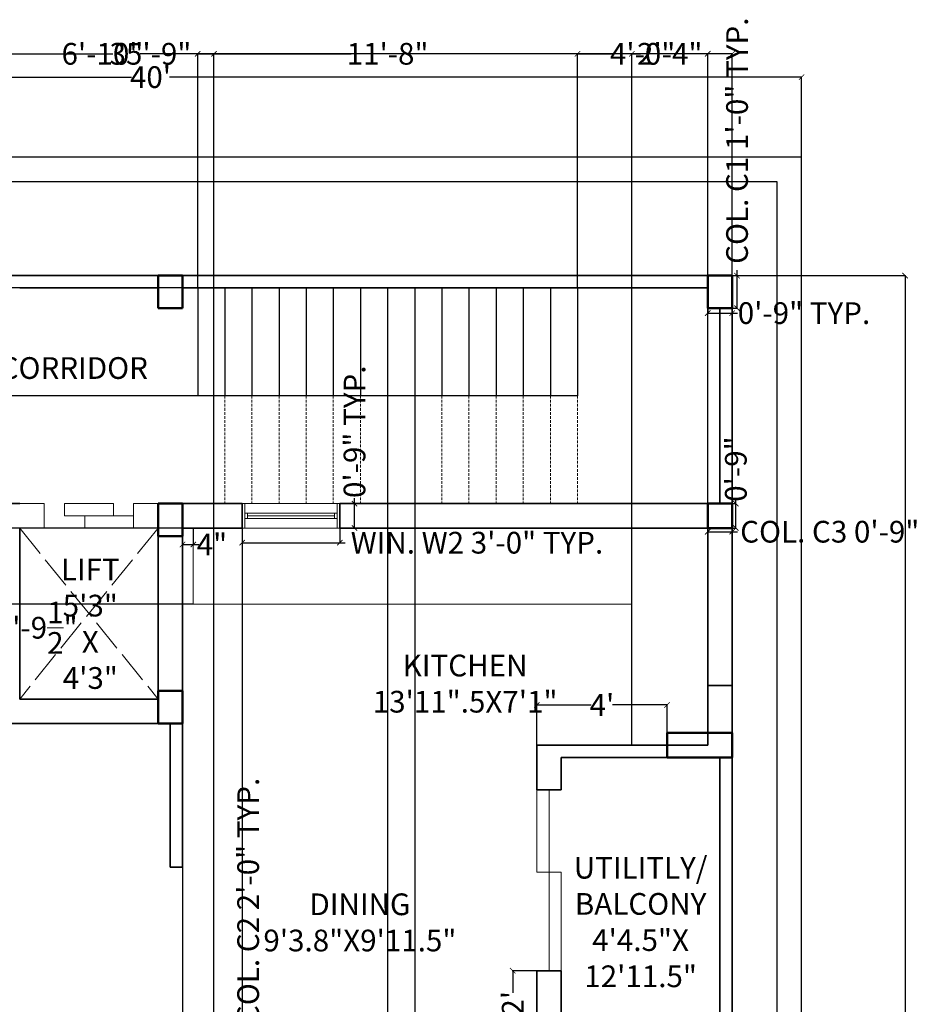
# Model space of a CAD drawing. Units: inches. Extents: x 490 to 1091, y 501 to 1322.
# Tile 5 of 5: x 759 to 1091, y 959 to 1322. Entities that reach past the tile are written whole.
import ezdxf

# ---------------------------------------------------------------- set-up
doc = ezdxf.new("R2010")
doc.units = ezdxf.units.IN
doc.header["$MEASUREMENT"] = 0
doc.linetypes.add('ACAD_ISO02W100', pattern=[15, 12, -3])
doc.linetypes.add('DASHEDX2', pattern=[1.5, 1, -0.5])
for name, color, linetype, lineweight in [('A-ANNO-DIMS', 2, 'Continuous', 18), ('A-AREA-IDEN', 7, 'Continuous', 25), ('A-COLS', 12, 'Continuous', 50), ('A-DOOR', 3, 'Continuous', 20), ('A-EQPM-EVTR', 152, 'Continuous', 20), ('A-EQPM-EVTR-HIDN', 152, 'ACAD_ISO02W100', 13), ('A-FLOR-FIXT', 8, 'Continuous', 20), ('A-FLOR-STRS', 12, 'Continuous', 25), ('A-FLOR-STRS-OVHD', 12, 'DASHEDX2', 18), ('A-GLAZ', 4, 'Continuous', 18), ('A-WALL', 7, 'Continuous', 35), ('C-PROP', 8, 'Continuous', 25)]:
    doc.layers.add(name, color=color, linetype=linetype, lineweight=lineweight)
doc.styles.get("Standard").update_dxf_attribs({"font": 'arial.ttf'})
doc.dimstyles.get("Standard").update_dxf_attribs({"dimtxt": 8, "dimasz": 2, "dimexe": 0.18, "dimexo": 0.0625, "dimgap": 0.09, "dimtad": 0, "dimdec": 1, "dimzin": 0, "dimdsep": 46, "dimlunit": 4, "dimtxsty": 'Standard', "dimblk": 'ARCHTICK', "dimcen": 0.09, "dimadec": 0, "dimazin": 0, "dimtfac": 1, "dimtdec": 1, "dimtofl": 0, "dimtmove": 0, "dimatfit": 3, "dimldrblk": 'ARCHTICK', "dimfxl": 1, "dimtolj": 1, "dimtzin": 0, "dimarcsym": 0})

# ---------------------------------------------------------------- blocks, each defined once
blk = doc.blocks.new('_ArchTick')
at = {"color": 0, "linetype": 'ByBlock', "const_width": 0.15}
blk.add_lwpolyline([(-0.5, -0.5), (0.5, 0.5)], dxfattribs=at)
blk = doc.blocks.new('*D3')
at = {"layer": 'A-ANNO-DIMS', "color": 0, "lineweight": -2, "transparency": 16777216}
for p, q in [((567.27, 1270.95), (567.27, 1300.61)), ((567.27, 1300.43), (800.23, 1300.43)), ((1047.27, 1300.43), (814.31, 1300.43)), ((1047.27, 1270.95), (1047.27, 1300.61))]:
    blk.add_line(p, q, dxfattribs=at)
at = {"layer": 'Defpoints', "color": 0, "transparency": 16777216}
for p in [(567.27, 1300.43), (567.27, 1270.88), (1047.27, 1270.88)]:
    blk.add_point(p, dxfattribs=at)
at = {"layer": 'A-ANNO-DIMS', "color": 0, "lineweight": -2, "transparency": 16777216, "xscale": 2, "yscale": 2, "zscale": 2, "rotation": 180}
blk.add_blockref('_ArchTick', (567.27, 1300.43), dxfattribs=at)
at = {"layer": 'A-ANNO-DIMS', "color": 0, "lineweight": -2, "transparency": 16777216, "xscale": 2, "yscale": 2, "zscale": 2}
blk.add_blockref('_ArchTick', (1047.27, 1300.43), dxfattribs=at)
at = {"layer": 'A-ANNO-DIMS', "color": 0, "transparency": 16777216, "insert": (807.27, 1300.43), "char_height": 8, "attachment_point": 5}
blk.add_mtext("\\A1;40'", dxfattribs=at)
blk = doc.blocks.new('jcjg  bmvh')
for p, q in [((1232.66, 1066.6), (1223.66, 1066.6)), ((1223.66, 1066.6), (1223.66, 1042.6)), ((1232.66, 1042.6), (1232.66, 1066.6)), ((1223.66, 1042.6), (1232.66, 1042.6))]:
    blk.add_line(p, q)
blk = doc.blocks.new('hcjfukik')
for p, q in [((1274.78, 1182.51), (1265.78, 1182.51)), ((1265.78, 1182.51), (1265.78, 1173.51)), ((1274.78, 1173.51), (1274.78, 1182.51)), ((1265.78, 1173.51), (1274.78, 1173.51))]:
    blk.add_line(p, q)
blk = doc.blocks.new('*D7')
at = {"layer": 'A-ANNO-DIMS', "color": 0, "lineweight": -2, "transparency": 16777216}
for p, q in [((949.67, 1054.35), (949.67, 1069.27)), ((949.67, 1069.09), (969.74, 1069.09)), ((997.67, 1069.09), (977.6, 1069.09)), ((997.67, 1054.35), (997.67, 1069.27))]:
    blk.add_line(p, q, dxfattribs=at)
at = {"layer": 'Defpoints', "color": 0, "transparency": 16777216}
for p in [(997.67, 1069.09), (949.67, 1054.28), (997.67, 1054.28)]:
    blk.add_point(p, dxfattribs=at)
at = {"layer": 'A-ANNO-DIMS', "color": 0, "lineweight": -2, "transparency": 16777216, "xscale": 2, "yscale": 2, "zscale": 2, "rotation": 180}
blk.add_blockref('_ArchTick', (949.67, 1069.09), dxfattribs=at)
at = {"layer": 'A-ANNO-DIMS', "color": 0, "lineweight": -2, "transparency": 16777216, "xscale": 2, "yscale": 2, "zscale": 2}
blk.add_blockref('_ArchTick', (997.67, 1069.09), dxfattribs=at)
at = {"layer": 'A-ANNO-DIMS', "color": 0, "transparency": 16777216, "insert": (973.67, 1069.09), "char_height": 8, "attachment_point": 5}
blk.add_mtext("\\A1;4'", dxfattribs=at)
blk = doc.blocks.new('*D13')
at = {"layer": 'A-ANNO-DIMS', "color": 0, "lineweight": -2, "transparency": 16777216}
for p, q in [((819.07, 1134.22), (819.07, 1128.05)), ((823.07, 1134.22), (823.07, 1128.05)), ((819.07, 1128.23), (823.07, 1128.23)), ((823.07, 1128.23), (825.07, 1128.23))]:
    blk.add_line(p, q, dxfattribs=at)
at = {"layer": 'Defpoints', "color": 0, "transparency": 16777216}
for p in [(819.07, 1134.28), (823.07, 1134.28), (823.07, 1128.23)]:
    blk.add_point(p, dxfattribs=at)
at = {"layer": 'A-ANNO-DIMS', "color": 0, "lineweight": -2, "transparency": 16777216, "xscale": 2, "yscale": 2, "zscale": 2, "rotation": 180}
blk.add_blockref('_ArchTick', (819.07, 1128.23), dxfattribs=at)
at = {"layer": 'A-ANNO-DIMS', "color": 0, "lineweight": -2, "transparency": 16777216, "xscale": 2, "yscale": 2, "zscale": 2}
blk.add_blockref('_ArchTick', (823.07, 1128.23), dxfattribs=at)
at = {"layer": 'A-ANNO-DIMS', "color": 0, "transparency": 16777216, "insert": (829.92, 1128.23), "char_height": 8, "attachment_point": 5}
blk.add_mtext('\\A1;4"', dxfattribs=at)
blk = doc.blocks.new('bnfgfhvhm')
for p, q in [((1106.43, 1203.63), (1115.43, 1203.63)), ((1106.43, 1191.63), (1106.43, 1203.63)), ((1115.43, 1203.63), (1115.43, 1191.63)), ((1115.43, 1191.63), (1106.43, 1191.63))]:
    blk.add_line(p, q)
blk = doc.blocks.new('fvbfbvc hbmh')
for p, q in [((1342.5, 1176.65), (1378.5, 1176.65)), ((1342.5, 1167.65), (1342.5, 1176.65)), ((1343.5, 1167.65), (1343.5, 1176.65)), ((1377.5, 1176.65), (1377.5, 1167.65)), ((1378.5, 1176.65), (1378.5, 1167.65)), ((1343.5, 1173.15), (1377.5, 1173.15)), ((1344.5, 1171.15), (1344.5, 1173.15)), ((1344.5, 1172.15), (1376.5, 1172.15)), ((1376.5, 1173.15), (1376.5, 1171.15)), ((1343.5, 1171.15), (1377.5, 1171.15)), ((1378.5, 1167.65), (1342.5, 1167.65))]:
    blk.add_line(p, q)
blk = doc.blocks.new('*D26')
at = {"layer": 'A-ANNO-DIMS', "color": 0, "lineweight": -2, "transparency": 16777216}
for p, q in [((728.47, 1134.22), (728.47, 1097.37)), ((750.07, 1134.22), (750.07, 1097.37)), ((728.47, 1097.55), (750.07, 1097.55)), ((750.07, 1097.55), (752.07, 1097.55))]:
    blk.add_line(p, q, dxfattribs=at)
at = {"layer": 'Defpoints', "color": 0, "transparency": 16777216}
for p in [(728.47, 1134.28), (750.07, 1134.28), (750.07, 1097.55)]:
    blk.add_point(p, dxfattribs=at)
at = {"layer": 'A-ANNO-DIMS', "color": 0, "lineweight": -2, "transparency": 16777216, "xscale": 2, "yscale": 2, "zscale": 2, "rotation": 180}
blk.add_blockref('_ArchTick', (728.47, 1097.55), dxfattribs=at)
at = {"layer": 'A-ANNO-DIMS', "color": 0, "lineweight": -2, "transparency": 16777216, "xscale": 2, "yscale": 2, "zscale": 2}
blk.add_blockref('_ArchTick', (750.07, 1097.55), dxfattribs=at)
at = {"layer": 'A-ANNO-DIMS', "color": 0, "transparency": 16777216, "insert": (765.33, 1097.55), "char_height": 8, "attachment_point": 5}
blk.add_mtext('\\A1;1\'-9{\\H1x;\\S1/2;}"', dxfattribs=at)
blk = doc.blocks.new('*D31')
at = {"layer": 'A-ANNO-DIMS', "color": 0, "lineweight": -2, "transparency": 16777216}
for p, q in [((949.61, 971.18), (940.6, 971.18)), ((940.78, 971.18), (940.78, 963.02)), ((940.78, 947.18), (940.78, 955.35)), ((949.61, 947.18), (940.6, 947.18))]:
    blk.add_line(p, q, dxfattribs=at)
at = {"layer": 'Defpoints', "color": 0, "transparency": 16777216}
for p in [(940.78, 971.18), (949.67, 971.18), (949.67, 947.18)]:
    blk.add_point(p, dxfattribs=at)
at = {"layer": 'A-ANNO-DIMS', "color": 0, "lineweight": -2, "transparency": 16777216, "xscale": 2, "yscale": 2, "zscale": 2}
for p, rotation in [((940.78, 971.18), 90), ((940.78, 947.18), 270)]:
    blk.add_blockref('_ArchTick', p, dxfattribs=dict(at, rotation=rotation))
at = {"layer": 'A-ANNO-DIMS', "color": 0, "transparency": 16777216, "insert": (940.78, 959.18), "char_height": 8, "attachment_point": 5, "rotation": 90}
blk.add_mtext("\\A1;2'", dxfattribs=at)
blk = doc.blocks.new('*D48')
at = {"layer": 'A-ANNO-DIMS', "color": 0, "lineweight": -2, "transparency": 16777216}
for p, q in [((1021.73, 1227.28), (1023.65, 1227.28)), ((1023.47, 1227.28), (1023.47, 1229.28)), ((1023.47, 1215.28), (1023.47, 1227.28)), ((1021.73, 1215.28), (1023.65, 1215.28))]:
    blk.add_line(p, q, dxfattribs=at)
at = {"layer": 'Defpoints', "color": 0, "transparency": 16777216}
for p in [(1021.67, 1227.28), (1023.47, 1227.28), (1021.67, 1215.28)]:
    blk.add_point(p, dxfattribs=at)
at = {"layer": 'A-ANNO-DIMS', "color": 0, "lineweight": -2, "transparency": 16777216, "xscale": 2, "yscale": 2, "zscale": 2}
for p, rotation in [((1023.47, 1227.28), 90), ((1023.47, 1215.28), 270)]:
    blk.add_blockref('_ArchTick', p, dxfattribs=dict(at, rotation=rotation))
at = {"layer": 'A-ANNO-DIMS', "color": 0, "transparency": 16777216, "insert": (1023.47, 1277), "char_height": 8, "attachment_point": 5, "rotation": 90}
blk.add_mtext('\\A1;COL. C1 1\'-0" TYP.', dxfattribs=at)
blk = doc.blocks.new('*D49')
at = {"layer": 'A-ANNO-DIMS', "color": 0, "lineweight": -2, "transparency": 16777216}
for p, q in [((1012.67, 1215.22), (1012.67, 1213.3)), ((1012.67, 1213.48), (1021.67, 1213.48)), ((1021.67, 1215.22), (1021.67, 1213.3)), ((1021.67, 1213.48), (1023.67, 1213.48))]:
    blk.add_line(p, q, dxfattribs=at)
at = {"layer": 'Defpoints', "color": 0, "transparency": 16777216}
for p in [(1012.67, 1215.28), (1021.67, 1215.28), (1021.67, 1213.48)]:
    blk.add_point(p, dxfattribs=at)
at = {"layer": 'A-ANNO-DIMS', "color": 0, "lineweight": -2, "transparency": 16777216, "xscale": 2, "yscale": 2, "zscale": 2, "rotation": 180}
blk.add_blockref('_ArchTick', (1012.67, 1213.48), dxfattribs=at)
at = {"layer": 'A-ANNO-DIMS', "color": 0, "lineweight": -2, "transparency": 16777216, "xscale": 2, "yscale": 2, "zscale": 2}
blk.add_blockref('_ArchTick', (1021.67, 1213.48), dxfattribs=at)
at = {"layer": 'A-ANNO-DIMS', "color": 0, "transparency": 16777216, "insert": (1048.14, 1213.48), "char_height": 8, "attachment_point": 5}
blk.add_mtext('\\A1;0\'-9" TYP.', dxfattribs=at)
blk = doc.blocks.new('*D50')
at = {"layer": 'A-ANNO-DIMS', "color": 0, "lineweight": -2, "transparency": 16777216}
for p, q in [((839.73, 947.18), (843.45, 947.18)), ((843.27, 947.18), (843.27, 949.18)), ((843.27, 923.18), (843.27, 947.18)), ((839.73, 923.18), (843.45, 923.18))]:
    blk.add_line(p, q, dxfattribs=at)
at = {"layer": 'Defpoints', "color": 0, "transparency": 16777216}
for p in [(839.67, 947.18), (843.27, 947.18), (839.67, 923.18)]:
    blk.add_point(p, dxfattribs=at)
at = {"layer": 'A-ANNO-DIMS', "color": 0, "lineweight": -2, "transparency": 16777216, "xscale": 2, "yscale": 2, "zscale": 2}
for p, rotation in [((843.27, 947.18), 90), ((843.27, 923.18), 270)]:
    blk.add_blockref('_ArchTick', p, dxfattribs=dict(at, rotation=rotation))
at = {"layer": 'A-ANNO-DIMS', "color": 0, "transparency": 16777216, "insert": (843.27, 996.9), "char_height": 8, "attachment_point": 5, "rotation": 90}
blk.add_mtext('\\A1;COL. C2 2\'-0" TYP.', dxfattribs=at)
blk = doc.blocks.new('*D52')
at = {"layer": 'A-ANNO-DIMS', "color": 0, "lineweight": -2, "transparency": 16777216}
for p, q in [((1012.67, 1134.22), (1012.67, 1132.75)), ((1012.67, 1132.93), (1021.67, 1132.93)), ((1021.67, 1134.22), (1021.67, 1132.75)), ((1021.67, 1132.93), (1023.67, 1132.93))]:
    blk.add_line(p, q, dxfattribs=at)
at = {"layer": 'Defpoints', "color": 0, "transparency": 16777216}
for p in [(1012.67, 1134.28), (1021.67, 1134.28), (1021.67, 1132.93)]:
    blk.add_point(p, dxfattribs=at)
at = {"layer": 'A-ANNO-DIMS', "color": 0, "lineweight": -2, "transparency": 16777216, "xscale": 2, "yscale": 2, "zscale": 2, "rotation": 180}
blk.add_blockref('_ArchTick', (1012.67, 1132.93), dxfattribs=at)
at = {"layer": 'A-ANNO-DIMS', "color": 0, "lineweight": -2, "transparency": 16777216, "xscale": 2, "yscale": 2, "zscale": 2}
blk.add_blockref('_ArchTick', (1021.67, 1132.93), dxfattribs=at)
at = {"layer": 'A-ANNO-DIMS', "color": 0, "transparency": 16777216, "insert": (1057.64, 1132.93), "char_height": 8, "attachment_point": 5}
blk.add_mtext('\\A1;COL. C3 0\'-9"', dxfattribs=at)
blk = doc.blocks.new('*D53')
at = {"layer": 'A-ANNO-DIMS', "color": 0, "lineweight": -2, "transparency": 16777216}
for p, q in [((1021.73, 1143.28), (1023.2, 1143.28)), ((1023.02, 1143.28), (1023.02, 1145.28)), ((1023.02, 1134.28), (1023.02, 1143.28)), ((1021.73, 1134.28), (1023.2, 1134.28))]:
    blk.add_line(p, q, dxfattribs=at)
at = {"layer": 'Defpoints', "color": 0, "transparency": 16777216}
for p in [(1021.67, 1143.28), (1023.02, 1143.28), (1021.67, 1134.28)]:
    blk.add_point(p, dxfattribs=at)
at = {"layer": 'A-ANNO-DIMS', "color": 0, "lineweight": -2, "transparency": 16777216, "xscale": 2, "yscale": 2, "zscale": 2}
for p, rotation in [((1023.02, 1143.28), 90), ((1023.02, 1134.28), 270)]:
    blk.add_blockref('_ArchTick', p, dxfattribs=dict(at, rotation=rotation))
at = {"layer": 'A-ANNO-DIMS', "color": 0, "transparency": 16777216, "insert": (1023.02, 1156.01), "char_height": 8, "attachment_point": 5, "rotation": 90}
blk.add_mtext('\\A1;0\'-9"', dxfattribs=at)
blk = doc.blocks.new('*D60')
at = {"layer": 'A-ANNO-DIMS', "color": 0, "lineweight": -2, "transparency": 16777216}
for p, q in [((841.07, 1134.22), (841.07, 1128.7)), ((877.07, 1134.22), (877.07, 1128.7)), ((841.07, 1128.88), (877.07, 1128.88)), ((877.07, 1128.88), (879.07, 1128.88))]:
    blk.add_line(p, q, dxfattribs=at)
at = {"layer": 'Defpoints', "color": 0, "transparency": 16777216}
for p in [(841.07, 1134.28), (877.07, 1134.28), (877.07, 1128.88)]:
    blk.add_point(p, dxfattribs=at)
at = {"layer": 'A-ANNO-DIMS', "color": 0, "lineweight": -2, "transparency": 16777216, "xscale": 2, "yscale": 2, "zscale": 2, "rotation": 180}
blk.add_blockref('_ArchTick', (841.07, 1128.88), dxfattribs=at)
at = {"layer": 'A-ANNO-DIMS', "color": 0, "lineweight": -2, "transparency": 16777216, "xscale": 2, "yscale": 2, "zscale": 2}
blk.add_blockref('_ArchTick', (877.07, 1128.88), dxfattribs=at)
at = {"layer": 'A-ANNO-DIMS', "color": 0, "transparency": 16777216, "insert": (927.61, 1128.88), "char_height": 8, "attachment_point": 5}
blk.add_mtext('\\A1;WIN. W2 3\'-0" TYP.', dxfattribs=at)
blk = doc.blocks.new('*D61')
at = {"layer": 'A-ANNO-DIMS', "color": 0, "lineweight": -2, "transparency": 16777216}
for p, q in [((877.13, 1143.28), (882.65, 1143.28)), ((882.47, 1143.28), (882.47, 1145.28)), ((882.47, 1134.28), (882.47, 1143.28)), ((877.13, 1134.28), (882.65, 1134.28))]:
    blk.add_line(p, q, dxfattribs=at)
at = {"layer": 'Defpoints', "color": 0, "transparency": 16777216}
for p in [(877.07, 1143.28), (882.47, 1143.28), (877.07, 1134.28)]:
    blk.add_point(p, dxfattribs=at)
at = {"layer": 'A-ANNO-DIMS', "color": 0, "lineweight": -2, "transparency": 16777216, "xscale": 2, "yscale": 2, "zscale": 2}
for p, rotation in [((882.47, 1143.28), 90), ((882.47, 1134.28), 270)]:
    blk.add_blockref('_ArchTick', p, dxfattribs=dict(at, rotation=rotation))
at = {"layer": 'A-ANNO-DIMS', "color": 0, "transparency": 16777216, "insert": (882.47, 1169.76), "char_height": 8, "attachment_point": 5, "rotation": 90}
blk.add_mtext('\\A1;0\'-9" TYP.', dxfattribs=at)
blk = doc.blocks.new('*D64')
at = {"layer": 'A-ANNO-DIMS', "color": 0, "lineweight": -2, "transparency": 16777216}
for p, q in [((592.87, 1227.35), (592.87, 1309.19)), ((592.87, 1309.01), (793.44, 1309.01)), ((1021.67, 1309.01), (821.1, 1309.01)), ((1021.67, 1227.35), (1021.67, 1309.19))]:
    blk.add_line(p, q, dxfattribs=at)
at = {"layer": 'Defpoints', "color": 0, "transparency": 16777216}
for p in [(1021.67, 1309.01), (592.87, 1227.28), (1021.67, 1227.28)]:
    blk.add_point(p, dxfattribs=at)
at = {"layer": 'A-ANNO-DIMS', "color": 0, "lineweight": -2, "transparency": 16777216, "xscale": 2, "yscale": 2, "zscale": 2, "rotation": 180}
blk.add_blockref('_ArchTick', (592.87, 1309.01), dxfattribs=at)
at = {"layer": 'A-ANNO-DIMS', "color": 0, "lineweight": -2, "transparency": 16777216, "xscale": 2, "yscale": 2, "zscale": 2}
blk.add_blockref('_ArchTick', (1021.67, 1309.01), dxfattribs=at)
at = {"layer": 'A-ANNO-DIMS', "color": 0, "transparency": 16777216, "insert": (807.27, 1309.01), "char_height": 8, "attachment_point": 5}
blk.add_mtext('\\A1;35\'-9"', dxfattribs=at)
blk = doc.blocks.new('*D65')
at = {"layer": 'A-ANNO-DIMS', "color": 0, "lineweight": -2, "transparency": 16777216}
for p, q in [((1021.73, 1227.28), (1085.58, 1227.28)), ((1085.4, 1227.28), (1085.4, 918.72)), ((1085.4, 582.48), (1085.4, 891.05)), ((1021.73, 582.48), (1085.58, 582.48))]:
    blk.add_line(p, q, dxfattribs=at)
at = {"layer": 'Defpoints', "color": 0, "transparency": 16777216}
for p in [(1021.67, 1227.28), (1085.4, 1227.28), (1021.67, 582.48)]:
    blk.add_point(p, dxfattribs=at)
at = {"layer": 'A-ANNO-DIMS', "color": 0, "lineweight": -2, "transparency": 16777216, "xscale": 2, "yscale": 2, "zscale": 2}
for p, rotation in [((1085.4, 1227.28), 90), ((1085.4, 582.48), 270)]:
    blk.add_blockref('_ArchTick', p, dxfattribs=dict(at, rotation=rotation))
at = {"layer": 'A-ANNO-DIMS', "color": 0, "transparency": 16777216, "insert": (1085.4, 904.88), "char_height": 8, "attachment_point": 5, "rotation": 90}
blk.add_mtext('\\A1;53\'-9"', dxfattribs=at)
blk = doc.blocks.new('*D67')
at = {"layer": 'A-ANNO-DIMS', "color": 0, "lineweight": -2, "transparency": 16777216}
for p, q in [((824.67, 1222.85), (824.67, 1309.19)), ((824.67, 1309.01), (881.22, 1309.01)), ((964.67, 1309.01), (908.12, 1309.01)), ((964.67, 1222.85), (964.67, 1309.19))]:
    blk.add_line(p, q, dxfattribs=at)
at = {"layer": 'Defpoints', "color": 0, "transparency": 16777216}
for p in [(964.67, 1309.01), (824.67, 1222.78), (964.67, 1222.78)]:
    blk.add_point(p, dxfattribs=at)
at = {"layer": 'A-ANNO-DIMS', "color": 0, "lineweight": -2, "transparency": 16777216, "xscale": 2, "yscale": 2, "zscale": 2, "rotation": 180}
blk.add_blockref('_ArchTick', (824.67, 1309.01), dxfattribs=at)
at = {"layer": 'A-ANNO-DIMS', "color": 0, "lineweight": -2, "transparency": 16777216, "xscale": 2, "yscale": 2, "zscale": 2}
blk.add_blockref('_ArchTick', (964.67, 1309.01), dxfattribs=at)
at = {"layer": 'A-ANNO-DIMS', "color": 0, "transparency": 16777216, "insert": (894.67, 1309.01), "char_height": 8, "attachment_point": 5}
blk.add_mtext('\\A1;11\'-8"', dxfattribs=at)
blk = doc.blocks.new('*D68')
at = {"layer": 'A-ANNO-DIMS', "color": 0, "lineweight": -2, "transparency": 16777216}
for p, q in [((964.67, 1222.85), (964.67, 1309.19)), ((964.67, 1309.01), (977.79, 1309.01)), ((1012.67, 1309.01), (999.55, 1309.01)), ((1012.67, 1222.85), (1012.67, 1309.19))]:
    blk.add_line(p, q, dxfattribs=at)
at = {"layer": 'Defpoints', "color": 0, "transparency": 16777216}
for p in [(1012.67, 1309.01), (964.67, 1222.78), (1012.67, 1222.78)]:
    blk.add_point(p, dxfattribs=at)
at = {"layer": 'A-ANNO-DIMS', "color": 0, "lineweight": -2, "transparency": 16777216, "xscale": 2, "yscale": 2, "zscale": 2, "rotation": 180}
blk.add_blockref('_ArchTick', (964.67, 1309.01), dxfattribs=at)
at = {"layer": 'A-ANNO-DIMS', "color": 0, "lineweight": -2, "transparency": 16777216, "xscale": 2, "yscale": 2, "zscale": 2}
blk.add_blockref('_ArchTick', (1012.67, 1309.01), dxfattribs=at)
at = {"layer": 'A-ANNO-DIMS', "color": 0, "transparency": 16777216, "insert": (988.67, 1309.01), "char_height": 8, "attachment_point": 5}
blk.add_mtext('\\A1;4\'-0"', dxfattribs=at)
blk = doc.blocks.new('*D69')
at = {"layer": 'A-ANNO-DIMS', "color": 0, "lineweight": -2, "transparency": 16777216}
for p, q in [((894.67, 1182.97), (894.67, 512.57)), ((904.67, 1182.97), (904.67, 512.57)), ((894.67, 512.75), (904.67, 512.75)), ((904.67, 512.75), (906.67, 512.75))]:
    blk.add_line(p, q, dxfattribs=at)
at = {"layer": 'Defpoints', "color": 0, "transparency": 16777216}
for p in [(894.67, 1183.03), (904.67, 1183.03), (904.67, 512.75)]:
    blk.add_point(p, dxfattribs=at)
at = {"layer": 'A-ANNO-DIMS', "color": 0, "lineweight": -2, "transparency": 16777216, "xscale": 2, "yscale": 2, "zscale": 2, "rotation": 180}
blk.add_blockref('_ArchTick', (894.67, 512.75), dxfattribs=at)
at = {"layer": 'A-ANNO-DIMS', "color": 0, "lineweight": -2, "transparency": 16777216, "xscale": 2, "yscale": 2, "zscale": 2}
blk.add_blockref('_ArchTick', (904.67, 512.75), dxfattribs=at)
at = {"layer": 'A-ANNO-DIMS', "color": 0, "transparency": 16777216, "insert": (920.5, 512.75), "char_height": 8, "attachment_point": 5}
blk.add_mtext('\\A1;0\'-10"', dxfattribs=at)
blk = doc.blocks.new('*D70')
at = {"layer": 'A-ANNO-DIMS', "color": 0, "lineweight": -2, "transparency": 16777216}
for p, q in [((824.61, 1222.78), (528.96, 1222.78)), ((529.14, 1222.78), (529.14, 1213.63)), ((529.14, 1183.03), (529.14, 1192.19)), ((824.61, 1183.03), (528.96, 1183.03))]:
    blk.add_line(p, q, dxfattribs=at)
at = {"layer": 'Defpoints', "color": 0, "transparency": 16777216}
for p in [(824.67, 1222.78), (529.14, 1183.03), (824.67, 1183.03)]:
    blk.add_point(p, dxfattribs=at)
at = {"layer": 'A-ANNO-DIMS', "color": 0, "lineweight": -2, "transparency": 16777216, "xscale": 2, "yscale": 2, "zscale": 2}
for p, rotation in [((529.14, 1222.78), 90), ((529.14, 1183.03), 270)]:
    blk.add_blockref('_ArchTick', p, dxfattribs=dict(at, rotation=rotation))
at = {"layer": 'A-ANNO-DIMS', "color": 0, "transparency": 16777216, "insert": (529.14, 1202.91), "char_height": 8, "attachment_point": 5, "rotation": 90}
blk.add_mtext('\\A1;3\'-4"', dxfattribs=at)
blk = doc.blocks.new('*D71')
at = {"layer": 'A-ANNO-DIMS', "color": 0, "lineweight": -2, "transparency": 16777216}
for p, q in [((819.07, 1134.22), (819.07, 512.57)), ((841.07, 1134.22), (841.07, 512.57)), ((819.07, 512.75), (841.07, 512.75)), ((841.07, 512.75), (843.07, 512.75))]:
    blk.add_line(p, q, dxfattribs=at)
at = {"layer": 'Defpoints', "color": 0, "transparency": 16777216}
for p in [(819.07, 1134.28), (841.07, 1134.28), (841.07, 512.75)]:
    blk.add_point(p, dxfattribs=at)
at = {"layer": 'A-ANNO-DIMS', "color": 0, "lineweight": -2, "transparency": 16777216, "xscale": 2, "yscale": 2, "zscale": 2, "rotation": 180}
blk.add_blockref('_ArchTick', (819.07, 512.75), dxfattribs=at)
at = {"layer": 'A-ANNO-DIMS', "color": 0, "lineweight": -2, "transparency": 16777216, "xscale": 2, "yscale": 2, "zscale": 2}
blk.add_blockref('_ArchTick', (841.07, 512.75), dxfattribs=at)
at = {"layer": 'A-ANNO-DIMS', "color": 0, "transparency": 16777216, "insert": (856.52, 512.75), "char_height": 8, "attachment_point": 5}
blk.add_mtext('\\A1;1\'-10"', dxfattribs=at)
blk = doc.blocks.new('*D72')
at = {"layer": 'A-ANNO-DIMS', "color": 0, "lineweight": -2, "transparency": 16777216}
for p, q in [((823.01, 1134.28), (528.96, 1134.28)), ((529.14, 1134.28), (529.14, 1131.08)), ((529.14, 1106.28), (529.14, 1109.49)), ((823.01, 1106.28), (528.96, 1106.28))]:
    blk.add_line(p, q, dxfattribs=at)
at = {"layer": 'Defpoints', "color": 0, "transparency": 16777216}
for p in [(823.07, 1134.28), (529.14, 1106.28), (823.07, 1106.28)]:
    blk.add_point(p, dxfattribs=at)
at = {"layer": 'A-ANNO-DIMS', "color": 0, "lineweight": -2, "transparency": 16777216, "xscale": 2, "yscale": 2, "zscale": 2}
for p, rotation in [((529.14, 1134.28), 90), ((529.14, 1106.28), 270)]:
    blk.add_blockref('_ArchTick', p, dxfattribs=dict(at, rotation=rotation))
at = {"layer": 'A-ANNO-DIMS', "color": 0, "transparency": 16777216, "insert": (529.14, 1120.28), "char_height": 8, "attachment_point": 5, "rotation": 90}
blk.add_mtext('\\A1;2\'-4"', dxfattribs=at)
blk = doc.blocks.new('*D73')
at = {"layer": 'A-ANNO-DIMS', "color": 0, "lineweight": -2, "transparency": 16777216}
for p, q in [((984.67, 1054.35), (984.67, 1309.19)), ((984.67, 1309.01), (987.88, 1309.01)), ((1012.67, 1309.01), (1009.46, 1309.01)), ((1012.67, 1054.35), (1012.67, 1309.19))]:
    blk.add_line(p, q, dxfattribs=at)
at = {"layer": 'Defpoints', "color": 0, "transparency": 16777216}
for p in [(1012.67, 1309.01), (984.67, 1054.28), (1012.67, 1054.28)]:
    blk.add_point(p, dxfattribs=at)
at = {"layer": 'A-ANNO-DIMS', "color": 0, "lineweight": -2, "transparency": 16777216, "xscale": 2, "yscale": 2, "zscale": 2, "rotation": 180}
blk.add_blockref('_ArchTick', (984.67, 1309.01), dxfattribs=at)
at = {"layer": 'A-ANNO-DIMS', "color": 0, "lineweight": -2, "transparency": 16777216, "xscale": 2, "yscale": 2, "zscale": 2}
blk.add_blockref('_ArchTick', (1012.67, 1309.01), dxfattribs=at)
at = {"layer": 'A-ANNO-DIMS', "color": 0, "transparency": 16777216, "insert": (998.67, 1309.01), "char_height": 8, "attachment_point": 5}
blk.add_mtext('\\A1;2\'-4"', dxfattribs=at)
blk = doc.blocks.new('*D76')
at = {"layer": 'A-ANNO-DIMS', "color": 0, "lineweight": -2, "transparency": 16777216}
for p, q in [((748.47, 802.15), (748.47, 1309.19)), ((748.47, 1309.01), (775.72, 1309.01)), ((830.67, 1309.01), (803.42, 1309.01)), ((830.67, 794.15), (830.67, 1309.19))]:
    blk.add_line(p, q, dxfattribs=at)
at = {"layer": 'Defpoints', "color": 0, "transparency": 16777216}
for p in [(830.67, 1309.01), (748.47, 802.08), (830.67, 794.08)]:
    blk.add_point(p, dxfattribs=at)
at = {"layer": 'A-ANNO-DIMS', "color": 0, "lineweight": -2, "transparency": 16777216, "xscale": 2, "yscale": 2, "zscale": 2, "rotation": 180}
blk.add_blockref('_ArchTick', (748.47, 1309.01), dxfattribs=at)
at = {"layer": 'A-ANNO-DIMS', "color": 0, "lineweight": -2, "transparency": 16777216, "xscale": 2, "yscale": 2, "zscale": 2}
blk.add_blockref('_ArchTick', (830.67, 1309.01), dxfattribs=at)
at = {"layer": 'A-ANNO-DIMS', "color": 0, "transparency": 16777216, "insert": (789.57, 1309.01), "char_height": 8, "attachment_point": 5}
blk.add_mtext('\\A1;6\'-10"', dxfattribs=at)

msp = doc.modelspace()

# ---------------------------------------------------------------- linework, layer by layer
at = {"layer": 'A-DOOR'}
for p, q in [((949.67, 1037.78), (949.67, 1007.48)), ((949.67, 1037.78), (954.17, 1037.78)), ((954.17, 1037.78), (954.17, 971.18)), ((949.67, 1007.48), (958.67, 1007.48)), ((958.67, 1007.48), (958.67, 971.18)), ((954.17, 971.18), (958.67, 971.18))]:
    msp.add_line(p, q, dxfattribs=at)
at = {"layer": 'A-EQPM-EVTR'}
for p, q in [((759.07, 1143.28), (768.07, 1143.28)), ((768.07, 1143.28), (768.07, 1134.28)), ((775.62, 1143.28), (793.62, 1143.28)), ((775.62, 1138.78), (775.62, 1143.28)), ((793.62, 1143.28), (793.62, 1138.78)), ((810.07, 1143.28), (801.07, 1143.28)), ((801.07, 1143.28), (801.07, 1134.28)), ((775.62, 1138.78), (801.07, 1138.78)), ((783.07, 1134.28), (783.07, 1138.78)), ((768.07, 1134.28), (759.07, 1134.28)), ((801.07, 1134.28), (783.07, 1134.28)), ((801.07, 1134.28), (810.07, 1134.28))]:
    msp.add_line(p, q, dxfattribs=at)
at = {"layer": 'A-EQPM-EVTR-HIDN'}
for p, q in [((759.07, 1134.28), (810.07, 1071.28)), ((810.07, 1134.28), (759.07, 1071.28))]:
    msp.add_line(p, q, dxfattribs=at)
at = {"layer": 'A-FLOR-FIXT'}
for p, q in [((823.07, 1134.28), (823.07, 1106.28)), ((823.07, 1106.28), (859.07, 1106.28)), ((859.07, 1106.28), (984.67, 1106.28)), ((984.67, 1054.28), (984.67, 1106.28))]:
    msp.add_line(p, q, dxfattribs=at)
at = {"layer": 'A-FLOR-STRS'}
for p, q in [((824.67, 1222.78), (824.67, 1183.03)), ((834.67, 1222.78), (834.67, 1183.03)), ((844.67, 1222.78), (844.67, 1183.03)), ((854.67, 1222.78), (854.67, 1183.03)), ((864.67, 1222.78), (864.67, 1183.03)), ((874.67, 1222.78), (874.67, 1183.03)), ((884.67, 1222.78), (884.67, 1183.03)), ((894.67, 1222.78), (894.67, 1183.03)), ((904.67, 1222.78), (904.67, 1183.03)), ((914.67, 1222.78), (914.67, 1183.03)), ((924.67, 1222.78), (924.67, 1183.03)), ((934.67, 1222.78), (934.67, 1183.03)), ((944.67, 1222.78), (944.67, 1183.03)), ((954.67, 1222.78), (954.67, 1183.03)), ((964.67, 1222.78), (964.67, 1183.03)), ((964.67, 1183.03), (824.67, 1183.03))]:
    msp.add_line(p, q, dxfattribs=at)
at = {"layer": 'A-FLOR-STRS-OVHD'}
for p, q in [((834.67, 1183.03), (834.67, 1143.28)), ((844.67, 1183.03), (844.67, 1143.28)), ((854.67, 1183.03), (854.67, 1143.28)), ((864.67, 1183.03), (864.67, 1143.28)), ((874.67, 1183.03), (874.67, 1143.28)), ((884.67, 1183.03), (884.67, 1143.28)), ((894.67, 1183.03), (894.67, 1143.28)), ((904.67, 1183.03), (904.67, 1143.28)), ((914.67, 1183.03), (914.67, 1143.28)), ((924.67, 1183.03), (924.67, 1143.28)), ((934.67, 1183.03), (934.67, 1143.28)), ((944.67, 1183.03), (944.67, 1143.28)), ((954.67, 1183.03), (954.67, 1143.28)), ((964.67, 1183.03), (964.67, 1143.28))]:
    msp.add_line(p, q, dxfattribs=at)
at = {"layer": 'A-WALL'}
for p, q in [((1021.67, 1227.28), (592.87, 1227.28)), ((1021.67, 791.58), (1021.67, 1227.28)), ((810.07, 1222.78), (759.07, 1222.78)), ((1012.67, 1222.78), (819.07, 1222.78)), ((1017.17, 1215.28), (1017.17, 1143.28)), ((759.07, 1143.28), (728.47, 1143.28)), ((841.07, 1143.28), (810.07, 1143.28)), ((819.07, 1134.28), (819.07, 1143.28)), ((841.07, 1134.28), (841.07, 1143.28)), ((1017.17, 1143.28), (877.07, 1143.28)), ((877.07, 1143.28), (877.07, 1134.28)), ((759.07, 1134.28), (759.07, 1071.28)), ((810.07, 1071.28), (810.07, 1134.28)), ((819.07, 1062.28), (819.07, 1134.28)), ((819.07, 1134.28), (823.07, 1134.28)), ((823.07, 1134.28), (841.07, 1134.28)), ((823.07, 1134.28), (841.07, 1134.28)), ((877.07, 1134.28), (1012.67, 1134.28)), ((1012.67, 1054.28), (1012.67, 1134.28)), ((1021.67, 1076.28), (1012.67, 1076.28)), ((759.07, 1071.28), (810.07, 1071.28)), ((750.07, 1062.28), (819.07, 1062.28)), ((814.57, 1062.28), (814.57, 1009.28)), ((819.07, 1009.28), (819.07, 1062.28)), ((1012.67, 1054.28), (949.67, 1054.28)), ((949.67, 1037.78), (949.67, 1054.28)), ((1012.67, 1049.78), (958.67, 1049.78)), ((958.67, 1049.78), (958.67, 1045.18)), ((958.67, 1049.78), (958.67, 1037.78)), ((1017.17, 1049.78), (1021.67, 1049.78)), ((1021.67, 1049.78), (1017.17, 1049.78)), ((1017.17, 1049.78), (1017.17, 791.58)), ((958.67, 1045.18), (958.67, 1037.78)), ((958.67, 1037.78), (949.67, 1037.78)), ((814.57, 1009.28), (819.07, 1009.28)), ((949.67, 947.18), (949.67, 971.18)), ((958.67, 971.18), (949.67, 971.18)), ((958.67, 971.18), (958.67, 947.18))]:
    msp.add_line(p, q, dxfattribs=at)
at = {"layer": 'C-PROP'}
for p, q in [((1047.27, 1270.88), (567.27, 1270.88)), ((1047.27, 550.88), (1047.27, 1270.88)), ((1038.27, 1261.88), (576.27, 1261.88)), ((1038.27, 559.88), (1038.27, 1261.88))]:
    msp.add_line(p, q, dxfattribs=at)

# ---------------------------------------------------------------- block references
at = {"layer": 'A-COLS'}
for name, p in [('bnfgfhvhm', (-296.36, 23.65)), ('bnfgfhvhm', (-93.76, 23.65)), ('bnfgfhvhm', (-296.36, -60.35)), ('hcjfukik', (-253.11, -39.23)), ('bnfgfhvhm', (-296.36, -129.35))]:
    msp.add_blockref(name, p, dxfattribs=at)
at = {"layer": 'A-COLS', "rotation": 90}
msp.add_blockref('jcjg  bmvh', (2064.27, -173.87), dxfattribs=at)
at = {"layer": 'A-GLAZ'}
msp.add_blockref('fvbfbvc hbmh', (-501.44, -33.36), dxfattribs=at)

# ---------------------------------------------------------------- texts
at = {"layer": 'A-AREA-IDEN', "char_height": 8, "attachment_point": 1}
for s, width, insert in [("\\pxqc;6'-7'.5  WIDE CORRIDOR", 135.1715, (678.87, 1197.24)), ('\\pxqc;LIFT \\P5\'3"\\PX\\P4\'3"', 44.7927, (762.7, 1123.04)), ('\\pxqc;KITCHEN \\P13\'11".5X7\'1"', 78.6246, (883.93, 1087.63)), ('\\pxqc;UTILITLY/\\PBALCONY\\P4\'4.5"X\\P12\'11.5"', 58.5, (958.67, 1013.13)), ('\\pxqc;DINING\\P9\'3.8"X9\'11.5"', 73.81, (847.56, 999.65))]:
    msp.add_mtext_dynamic_manual_height_columns(s, width=width, gutter_width=40, heights=[0], dxfattribs=dict(at, insert=insert))

# ---------------------------------------------------------------- dimensions: what is measured, and where the dimension line sits
at = {"layer": 'A-ANNO-DIMS'}
for base, p1, p2, text, picture, middle in [((1023.47, 1227.28), (1021.67, 1215.28), (1021.67, 1227.28), 'COL. C1 <> TYP.', '*D48', (1023.47, 1277)), ((882.47, 1143.28), (877.07, 1134.28), (877.07, 1143.28), '<> TYP.', '*D61', (882.47, 1169.76)), ((843.27, 947.18), (839.67, 923.18), (839.67, 947.18), 'COL. C2 <> TYP.', '*D50', (843.27, 996.9))]:
    dim = msp.add_linear_dim(base=base, p1=p1, p2=p2, angle=90, text=text, dimstyle='Standard', override={"dimdec": 1, "dimlfac": 1, "dimrnd": 0, "dimzin": 1, "dimdsep": 46, "dimlunit": 4, "dimfrac": 2}, dxfattribs=at)
    dim.commit()
    dim.dimension.update_dxf_attribs({"geometry": picture, "text_midpoint": middle})
for base, p1, p2, override, picture, middle in [((1021.67, 1309.01), (592.87, 1227.28), (1021.67, 1227.28), {"dimdec": 1, "dimlfac": 1, "dimrnd": 0, "dimzin": 1, "dimdsep": 46, "dimlunit": 4, "dimfrac": 2}, '*D64', (807.27, 1309.01)), ((830.67, 1309.01), (748.47, 802.08), (830.67, 794.08), {"dimdec": 1, "dimlfac": 1, "dimrnd": 0, "dimzin": 1, "dimdsep": 46, "dimlunit": 4, "dimfrac": 2}, '*D76', (789.57, 1309.01)), ((964.67, 1309.01), (824.67, 1222.78), (964.67, 1222.78), {"dimdec": 1, "dimlfac": 1, "dimrnd": 0, "dimzin": 1, "dimdsep": 46, "dimlunit": 4, "dimfrac": 2}, '*D67', (894.67, 1309.01)), ((1012.67, 1309.01), (964.67, 1222.78), (1012.67, 1222.78), {"dimdec": 1, "dimlfac": 1, "dimrnd": 0, "dimzin": 1, "dimdsep": 46, "dimlunit": 4, "dimfrac": 2}, '*D68', (988.67, 1309.01)), ((1012.67, 1309.01), (984.67, 1054.28), (1012.67, 1054.28), {"dimdec": 1, "dimlfac": 1, "dimrnd": 0, "dimzin": 1, "dimdsep": 46, "dimlunit": 4, "dimfrac": 2}, '*D73', (998.67, 1309.01)), ((567.27, 1300.43), (1047.27, 1270.88), (567.27, 1270.88), {"dimclrd": 0, "dimclre": 0, "dimclrt": 0}, '*D3', (807.27, 1300.43)), ((904.67, 512.75), (894.67, 1183.03), (904.67, 1183.03), {"dimdec": 1, "dimlfac": 1, "dimrnd": 0, "dimzin": 1, "dimdsep": 46, "dimlunit": 4, "dimfrac": 2}, '*D69', (920.5, 512.75)), ((750.07, 1097.55), (728.47, 1134.28), (750.07, 1134.28), {"dimclrd": 0, "dimclre": 0, "dimclrt": 0}, '*D26', (765.33, 1097.55)), ((823.07, 1128.23), (819.07, 1134.28), (823.07, 1134.28), {"dimclrd": 0, "dimclre": 0, "dimclrt": 0}, '*D13', (829.92, 1128.23)), ((841.07, 512.75), (819.07, 1134.28), (841.07, 1134.28), {"dimdec": 1, "dimlfac": 1, "dimrnd": 0, "dimzin": 1, "dimdsep": 46, "dimlunit": 4, "dimfrac": 2}, '*D71', (856.52, 512.75)), ((997.67, 1069.09), (949.67, 1054.28), (997.67, 1054.28), {"dimclrd": 0, "dimclre": 0, "dimclrt": 0}, '*D7', (973.67, 1069.09))]:
    dim = msp.add_linear_dim(base=base, p1=p1, p2=p2, dimstyle='Standard', override=override, dxfattribs=at)
    dim.commit()
    dim.dimension.update_dxf_attribs({"geometry": picture, "text_midpoint": middle})
for base, p1, p2, override, picture, middle in [((1085.4, 1227.28), (1021.67, 582.48), (1021.67, 1227.28), {"dimdec": 1, "dimlfac": 1, "dimrnd": 0, "dimzin": 1, "dimdsep": 46, "dimlunit": 4, "dimfrac": 2}, '*D65', (1085.4, 904.88)), ((529.139808, 1183.034783), (824.669808, 1222.784783), (824.669808, 1183.034783), {"dimdec": 1, "dimlfac": 1, "dimrnd": 0, "dimzin": 1, "dimdsep": 46, "dimlunit": 4, "dimfrac": 2}, '*D70', (529.139808, 1202.909783)), ((1023.02, 1143.28), (1021.67, 1134.28), (1021.67, 1143.28), {"dimdec": 1, "dimlfac": 1, "dimrnd": 0, "dimzin": 1, "dimdsep": 46, "dimlunit": 4, "dimfrac": 2}, '*D53', (1023.02, 1156.01)), ((529.14, 1106.28), (823.07, 1134.28), (823.07, 1106.28), {"dimdec": 1, "dimlfac": 1, "dimrnd": 0, "dimzin": 1, "dimdsep": 46, "dimlunit": 4, "dimfrac": 2}, '*D72', (529.14, 1120.28)), ((940.78, 971.18), (949.67, 947.18), (949.67, 971.18), {"dimclrd": 0, "dimclre": 0, "dimclrt": 0}, '*D31', (940.78, 959.18))]:
    dim = msp.add_linear_dim(base=base, p1=p1, p2=p2, angle=90, dimstyle='Standard', override=override, dxfattribs=at)
    dim.commit()
    dim.dimension.update_dxf_attribs({"geometry": picture, "text_midpoint": middle})
for base, p1, p2, text, picture, middle in [((1021.67, 1213.48), (1012.67, 1215.28), (1021.67, 1215.28), '<> TYP.', '*D49', (1048.14, 1213.48)), ((877.07, 1128.88), (841.07, 1134.28), (877.07, 1134.28), 'WIN. W2 <> TYP.', '*D60', (927.61, 1128.88)), ((1021.67, 1132.93), (1012.67, 1134.28), (1021.67, 1134.28), 'COL. C3 <>', '*D52', (1057.64, 1132.93))]:
    dim = msp.add_linear_dim(base=base, p1=p1, p2=p2, text=text, dimstyle='Standard', override={"dimdec": 1, "dimlfac": 1, "dimrnd": 0, "dimzin": 1, "dimdsep": 46, "dimlunit": 4, "dimfrac": 2}, dxfattribs=at)
    dim.commit()
    dim.dimension.update_dxf_attribs({"geometry": picture, "text_midpoint": middle})

doc.saveas('drawing.dxf')
